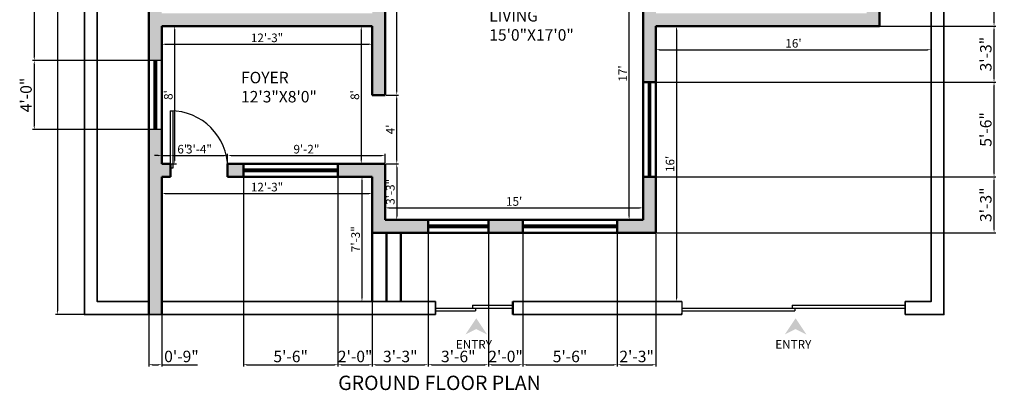
# Model space of a CAD drawing. Units: inches. Extents: x 2442 to 3851, y 589 to 2836.
# Tile 13 of 22: x 2448 to 3136, y 2138 to 2397. Entities that reach past the tile are written whole.
import ezdxf

# ---------------------------------------------------------------- set-up
doc = ezdxf.new("R2010")
doc.units = ezdxf.units.IN
for name, color, linetype, lineweight in [('A-ANNO-DIMS', 2, 'Continuous', 18), ('A-ANNO-SYMB', 1, 'Continuous', 18), ('A-ANNO-TEXT', 7, 'Continuous', 18), ('A-AREA-IDEN', 7, 'Continuous', 18), ('A-DOOR', 4, 'Continuous', 25), ('A-GLAZ', 1, 'Continuous', 25), ('A-WALL', 7, 'Continuous', 50), ('A-WALL-PATT', 8, 'Continuous', 13), ('C-PROP', 7, 'Continuous', 35)]:
    doc.layers.add(name, color=color, linetype=linetype, lineweight=lineweight)
doc.styles.get("Standard").update_dxf_attribs({"font": 'arial.ttf'})
doc.dimstyles.new('ISO-25', dxfattribs={"dimtxt": 8, "dimasz": 2.5, "dimexe": 1.25, "dimexo": 0.625, "dimtad": 1, "dimlunit": 3, "dimtxsty": 'Standard', "dimcen": 2.5, "dimadec": 0, "dimazin": 0, "dimtfac": 1, "dimtmove": 0, "dimatfit": 3, "dimfxl": 1, "dimarcsym": 0})

# ---------------------------------------------------------------- blocks, each defined once
blk = doc.blocks.new('*U22')
for p, q in [((0, 0), (0, -6)), ((40, 0), (40, -6))]:
    blk.add_line(p, q)
blk.add_lwpolyline([(0, 0), (0, 40), (1.75, 40), (1.75, 0)], close=True)
blk.add_arc((0, 0), 40, 0, 90)
blk = doc.blocks.new('*D36')
at = {"layer": 'A-ANNO-DIMS', "color": 0, "lineweight": -2, "transparency": 16777216}
for p, q in [((2492.97, 2791.21), (2473.47, 2791.21)), ((2474.72, 2788.71), (2474.72, 2193.71)), ((2492.97, 2191.21), (2473.47, 2191.21))]:
    blk.add_line(p, q, dxfattribs=at)
at = {"layer": 'A-ANNO-DIMS', "color": 0, "transparency": 16777216}
for points in [[(2474.3, 2788.71), (2475.14, 2788.71), (2474.72, 2791.21)], [(2474.3, 2193.71), (2475.14, 2193.71), (2474.72, 2191.21)]]:
    blk.add_solid(points, dxfattribs=at)
at = {"layer": 'Defpoints', "color": 0, "transparency": 16777216}
for p in [(2493.6, 2791.21), (2474.72, 2191.21), (2493.6, 2191.21)]:
    blk.add_point(p, dxfattribs=at)
at = {"layer": 'A-ANNO-DIMS', "color": 0, "transparency": 16777216, "insert": (2470.01, 2491.21), "char_height": 8, "attachment_point": 5, "rotation": 90}
blk.add_mtext("50'", dxfattribs=at)
blk = doc.blocks.new('*D54')
at = {"layer": 'A-ANNO-DIMS', "color": 0, "lineweight": -2, "transparency": 16777216}
for p, q in [((2703.6, 2257.83), (2703.6, 2266.79)), ((2706.1, 2265.54), (2881.1, 2265.54)), ((2883.6, 2257.83), (2883.6, 2266.79))]:
    blk.add_line(p, q, dxfattribs=at)
at = {"layer": 'A-ANNO-DIMS', "color": 0, "transparency": 16777216}
for points in [[(2706.1, 2265.96), (2706.1, 2265.13), (2703.6, 2265.54)], [(2881.1, 2265.96), (2881.1, 2265.13), (2883.6, 2265.54)]]:
    blk.add_solid(points, dxfattribs=at)
at = {"layer": 'Defpoints', "color": 0, "transparency": 16777216}
for p in [(2883.6, 2265.54), (2703.6, 2257.21), (2883.6, 2257.21)]:
    blk.add_point(p, dxfattribs=at)
at = {"layer": 'A-ANNO-DIMS', "color": 0, "transparency": 16777216, "insert": (2793.6, 2269.23), "char_height": 6, "attachment_point": 5}
blk.add_mtext("15'", dxfattribs=at)
blk = doc.blocks.new('*D55')
at = {"layer": 'A-ANNO-DIMS', "color": 0, "lineweight": -2, "transparency": 16777216}
for p, q in [((2882.97, 2461.21), (2872.6, 2461.21)), ((2873.85, 2259.71), (2873.85, 2458.71)), ((2882.97, 2257.21), (2872.6, 2257.21))]:
    blk.add_line(p, q, dxfattribs=at)
at = {"layer": 'A-ANNO-DIMS', "color": 0, "transparency": 16777216}
for points in [[(2873.44, 2458.71), (2874.27, 2458.71), (2873.85, 2461.21)], [(2873.44, 2259.71), (2874.27, 2259.71), (2873.85, 2257.21)]]:
    blk.add_solid(points, dxfattribs=at)
at = {"layer": 'Defpoints', "color": 0, "transparency": 16777216}
for p in [(2873.85, 2461.21), (2883.6, 2461.21), (2883.6, 2257.21)]:
    blk.add_point(p, dxfattribs=at)
at = {"layer": 'A-ANNO-DIMS', "color": 0, "transparency": 16777216, "insert": (2870.22, 2359.21), "char_height": 6, "attachment_point": 5, "rotation": 90}
blk.add_mtext("17'", dxfattribs=at)
blk = doc.blocks.new('*D58')
at = {"layer": 'A-ANNO-DIMS', "color": 0, "lineweight": -2, "transparency": 16777216}
for p, q in [((2547.6, 2391.58), (2547.6, 2378.36)), ((2694.6, 2391.58), (2694.6, 2378.36)), ((2550.1, 2379.61), (2692.1, 2379.61))]:
    blk.add_line(p, q, dxfattribs=at)
at = {"layer": 'A-ANNO-DIMS', "color": 0, "transparency": 16777216}
for points in [[(2550.1, 2380.03), (2550.1, 2379.19), (2547.6, 2379.61)], [(2692.1, 2380.03), (2692.1, 2379.19), (2694.6, 2379.61)]]:
    blk.add_solid(points, dxfattribs=at)
at = {"layer": 'Defpoints', "color": 0, "transparency": 16777216}
for p in [(2547.6, 2392.21), (2694.6, 2392.21), (2694.6, 2379.61)]:
    blk.add_point(p, dxfattribs=at)
at = {"layer": 'A-ANNO-DIMS', "color": 0, "transparency": 16777216, "insert": (2621.1, 2383.3), "char_height": 6, "attachment_point": 5}
blk.add_mtext('12\'-3"', dxfattribs=at)
blk = doc.blocks.new('*D59')
at = {"layer": 'A-ANNO-DIMS', "color": 0, "lineweight": -2, "transparency": 16777216}
for p, q in [((2693.97, 2392.21), (2685.61, 2392.21)), ((2686.86, 2389.71), (2686.86, 2298.71)), ((2693.97, 2296.21), (2685.61, 2296.21))]:
    blk.add_line(p, q, dxfattribs=at)
at = {"layer": 'A-ANNO-DIMS', "color": 0, "transparency": 16777216}
for points in [[(2686.44, 2389.71), (2687.27, 2389.71), (2686.86, 2392.21)], [(2686.44, 2298.71), (2687.27, 2298.71), (2686.86, 2296.21)]]:
    blk.add_solid(points, dxfattribs=at)
at = {"layer": 'Defpoints', "color": 0, "transparency": 16777216}
for p in [(2694.6, 2392.21), (2686.86, 2296.21), (2694.6, 2296.21)]:
    blk.add_point(p, dxfattribs=at)
at = {"layer": 'A-ANNO-DIMS', "color": 0, "transparency": 16777216, "insert": (2683.17, 2344.21), "char_height": 6, "attachment_point": 5, "rotation": 90}
blk.add_mtext("8'", dxfattribs=at)
blk = doc.blocks.new('*D77')
at = {"layer": 'A-ANNO-DIMS', "color": 0, "lineweight": -2, "transparency": 16777216}
for p, q in [((2548.22, 2392.21), (2557.88, 2392.21)), ((2556.63, 2298.71), (2556.63, 2389.71)), ((2548.22, 2296.21), (2557.88, 2296.21))]:
    blk.add_line(p, q, dxfattribs=at)
at = {"layer": 'A-ANNO-DIMS', "color": 0, "transparency": 16777216}
for points in [[(2556.21, 2389.71), (2557.05, 2389.71), (2556.63, 2392.21)], [(2556.21, 2298.71), (2557.05, 2298.71), (2556.63, 2296.21)]]:
    blk.add_solid(points, dxfattribs=at)
at = {"layer": 'Defpoints', "color": 0, "transparency": 16777216}
for p in [(2547.6, 2392.21), (2556.63, 2392.21), (2547.6, 2296.21)]:
    blk.add_point(p, dxfattribs=at)
at = {"layer": 'A-ANNO-DIMS', "color": 0, "transparency": 16777216, "insert": (2552.94, 2344.21), "char_height": 6, "attachment_point": 5, "rotation": 90}
blk.add_mtext("8'", dxfattribs=at)
blk = doc.blocks.new('*D78')
at = {"layer": 'A-ANNO-DIMS', "color": 0, "lineweight": -2, "transparency": 16777216}
for p, q in [((2547.6, 2296.83), (2547.6, 2303.24)), ((2553.6, 2296.83), (2553.6, 2303.24)), ((2545.1, 2301.99), (2542.6, 2301.99)), ((2547.6, 2301.99), (2553.6, 2301.99)), ((2556.1, 2301.99), (2566.78, 2301.99))]:
    blk.add_line(p, q, dxfattribs=at)
at = {"layer": 'A-ANNO-DIMS', "color": 0, "transparency": 16777216}
for points in [[(2545.1, 2302.41), (2545.1, 2301.58), (2547.6, 2301.99)], [(2556.1, 2302.41), (2556.1, 2301.58), (2553.6, 2301.99)]]:
    blk.add_solid(points, dxfattribs=at)
at = {"layer": 'Defpoints', "color": 0, "transparency": 16777216}
for p in [(2547.6, 2296.21), (2553.6, 2301.99), (2553.6, 2296.21)]:
    blk.add_point(p, dxfattribs=at)
at = {"layer": 'A-ANNO-DIMS', "color": 0, "transparency": 16777216, "insert": (2562.69, 2305.68), "char_height": 6, "attachment_point": 5}
blk.add_mtext('6"', dxfattribs=at)
blk = doc.blocks.new('*D79')
at = {"layer": 'A-ANNO-DIMS', "color": 0, "lineweight": -2, "transparency": 16777216}
for p, q in [((2553.6, 2296.83), (2553.6, 2303.24)), ((2593.6, 2296.83), (2593.6, 2303.24)), ((2556.1, 2301.99), (2591.1, 2301.99))]:
    blk.add_line(p, q, dxfattribs=at)
at = {"layer": 'A-ANNO-DIMS', "color": 0, "transparency": 16777216}
for points in [[(2556.1, 2302.41), (2556.1, 2301.58), (2553.6, 2301.99)], [(2591.1, 2302.41), (2591.1, 2301.58), (2593.6, 2301.99)]]:
    blk.add_solid(points, dxfattribs=at)
at = {"layer": 'Defpoints', "color": 0, "transparency": 16777216}
for p in [(2553.6, 2296.21), (2593.6, 2301.99), (2593.6, 2296.21)]:
    blk.add_point(p, dxfattribs=at)
at = {"layer": 'A-ANNO-DIMS', "color": 0, "transparency": 16777216, "insert": (2573.6, 2305.68), "char_height": 6, "attachment_point": 5}
blk.add_mtext('3\'-4"', dxfattribs=at)
blk = doc.blocks.new('*D80')
at = {"layer": 'A-ANNO-DIMS', "color": 0, "lineweight": -2, "transparency": 16777216}
for p, q in [((2593.6, 2296.83), (2593.6, 2303.24)), ((2703.6, 2296.83), (2703.6, 2303.24)), ((2596.1, 2301.99), (2701.1, 2301.99))]:
    blk.add_line(p, q, dxfattribs=at)
at = {"layer": 'A-ANNO-DIMS', "color": 0, "transparency": 16777216}
for points in [[(2596.1, 2302.41), (2596.1, 2301.58), (2593.6, 2301.99)], [(2701.1, 2302.41), (2701.1, 2301.58), (2703.6, 2301.99)]]:
    blk.add_solid(points, dxfattribs=at)
at = {"layer": 'Defpoints', "color": 0, "transparency": 16777216}
for p in [(2593.6, 2296.21), (2703.6, 2301.99), (2703.6, 2296.21)]:
    blk.add_point(p, dxfattribs=at)
at = {"layer": 'A-ANNO-DIMS', "color": 0, "transparency": 16777216, "insert": (2648.6, 2305.68), "char_height": 6, "attachment_point": 5}
blk.add_mtext('9\'-2"', dxfattribs=at)
blk = doc.blocks.new('*D81')
at = {"layer": 'A-ANNO-DIMS', "color": 0, "lineweight": -2, "transparency": 16777216}
for p, q in [((2704.22, 2296.21), (2712.89, 2296.21)), ((2711.64, 2293.71), (2711.64, 2259.71)), ((2704.22, 2257.21), (2712.89, 2257.21))]:
    blk.add_line(p, q, dxfattribs=at)
at = {"layer": 'A-ANNO-DIMS', "color": 0, "transparency": 16777216}
for points in [[(2711.22, 2293.71), (2712.05, 2293.71), (2711.64, 2296.21)], [(2711.22, 2259.71), (2712.05, 2259.71), (2711.64, 2257.21)]]:
    blk.add_solid(points, dxfattribs=at)
at = {"layer": 'Defpoints', "color": 0, "transparency": 16777216}
for p in [(2703.6, 2296.21), (2703.6, 2257.21), (2711.64, 2257.21)]:
    blk.add_point(p, dxfattribs=at)
at = {"layer": 'A-ANNO-DIMS', "color": 0, "transparency": 16777216, "insert": (2707.95, 2276.71), "char_height": 6, "attachment_point": 5, "rotation": 90}
blk.add_mtext('3\'-3"', dxfattribs=at)
blk = doc.blocks.new('*D82')
at = {"layer": 'A-ANNO-DIMS', "color": 0, "lineweight": -2, "transparency": 16777216}
for p, q in [((2704.22, 2344.21), (2712.89, 2344.21)), ((2711.64, 2298.71), (2711.64, 2341.71)), ((2704.22, 2296.21), (2712.89, 2296.21))]:
    blk.add_line(p, q, dxfattribs=at)
at = {"layer": 'A-ANNO-DIMS', "color": 0, "transparency": 16777216}
for points in [[(2711.22, 2341.71), (2712.05, 2341.71), (2711.64, 2344.21)], [(2711.22, 2298.71), (2712.05, 2298.71), (2711.64, 2296.21)]]:
    blk.add_solid(points, dxfattribs=at)
at = {"layer": 'Defpoints', "color": 0, "transparency": 16777216}
for p in [(2703.6, 2344.21), (2711.64, 2344.21), (2703.6, 2296.21)]:
    blk.add_point(p, dxfattribs=at)
at = {"layer": 'A-ANNO-DIMS', "color": 0, "transparency": 16777216, "insert": (2708.01, 2320.21), "char_height": 6, "attachment_point": 5, "rotation": 90}
blk.add_mtext("4'", dxfattribs=at)
blk = doc.blocks.new('*D83')
at = {"layer": 'A-ANNO-DIMS', "color": 0, "lineweight": -2, "transparency": 16777216}
for p, q in [((2704.22, 2506.21), (2712.89, 2506.21)), ((2711.64, 2346.71), (2711.64, 2503.71)), ((2704.22, 2344.21), (2712.89, 2344.21))]:
    blk.add_line(p, q, dxfattribs=at)
at = {"layer": 'A-ANNO-DIMS', "color": 0, "transparency": 16777216}
for points in [[(2711.22, 2503.71), (2712.05, 2503.71), (2711.64, 2506.21)], [(2711.22, 2346.71), (2712.05, 2346.71), (2711.64, 2344.21)]]:
    blk.add_solid(points, dxfattribs=at)
at = {"layer": 'Defpoints', "color": 0, "transparency": 16777216}
for p in [(2703.6, 2506.21), (2711.64, 2506.21), (2703.6, 2344.21)]:
    blk.add_point(p, dxfattribs=at)
at = {"layer": 'A-ANNO-DIMS', "color": 0, "transparency": 16777216, "insert": (2707.95, 2425.21), "char_height": 6, "attachment_point": 5, "rotation": 90}
blk.add_mtext('13\'-6"', dxfattribs=at)
blk = doc.blocks.new('*D89')
at = {"layer": 'A-ANNO-DIMS', "color": 0, "lineweight": -2, "transparency": 16777216}
for p, q in [((2892.6, 2391.58), (2892.6, 2374.53)), ((3084.6, 2391.58), (3084.6, 2374.53)), ((2895.1, 2375.78), (3082.1, 2375.78))]:
    blk.add_line(p, q, dxfattribs=at)
at = {"layer": 'A-ANNO-DIMS', "color": 0, "transparency": 16777216}
for points in [[(2895.1, 2376.2), (2895.1, 2375.37), (2892.6, 2375.78)], [(3082.1, 2376.2), (3082.1, 2375.37), (3084.6, 2375.78)]]:
    blk.add_solid(points, dxfattribs=at)
at = {"layer": 'Defpoints', "color": 0, "transparency": 16777216}
for p in [(2892.6, 2392.21), (3084.6, 2392.21), (3084.6, 2375.78)]:
    blk.add_point(p, dxfattribs=at)
at = {"layer": 'A-ANNO-DIMS', "color": 0, "transparency": 16777216, "insert": (2988.6, 2379.47), "char_height": 6, "attachment_point": 5}
blk.add_mtext("16'", dxfattribs=at)
blk = doc.blocks.new('*D90')
at = {"layer": 'A-ANNO-DIMS', "color": 0, "lineweight": -2, "transparency": 16777216}
for p, q in [((2893.22, 2392.21), (2908.16, 2392.21)), ((2906.91, 2389.71), (2906.91, 2202.71)), ((2893.22, 2200.21), (2908.16, 2200.21))]:
    blk.add_line(p, q, dxfattribs=at)
at = {"layer": 'A-ANNO-DIMS', "color": 0, "transparency": 16777216}
for points in [[(2906.5, 2389.71), (2907.33, 2389.71), (2906.91, 2392.21)], [(2906.5, 2202.71), (2907.33, 2202.71), (2906.91, 2200.21)]]:
    blk.add_solid(points, dxfattribs=at)
at = {"layer": 'Defpoints', "color": 0, "transparency": 16777216}
for p in [(2892.6, 2392.21), (2892.6, 2200.21), (2906.91, 2200.21)]:
    blk.add_point(p, dxfattribs=at)
at = {"layer": 'A-ANNO-DIMS', "color": 0, "transparency": 16777216, "insert": (2903.22, 2296.21), "char_height": 6, "attachment_point": 5, "rotation": 90}
blk.add_mtext("16'", dxfattribs=at)
blk = doc.blocks.new('*D91')
at = {"layer": 'A-ANNO-DIMS', "color": 0, "lineweight": -2, "transparency": 16777216}
for p, q in [((2694.6, 2286.58), (2694.6, 2274.29)), ((2547.6, 2277.87), (2547.6, 2274.29)), ((2550.1, 2275.54), (2692.1, 2275.54))]:
    blk.add_line(p, q, dxfattribs=at)
at = {"layer": 'A-ANNO-DIMS', "color": 0, "transparency": 16777216}
for points in [[(2550.1, 2275.95), (2550.1, 2275.12), (2547.6, 2275.54)], [(2692.1, 2275.95), (2692.1, 2275.12), (2694.6, 2275.54)]]:
    blk.add_solid(points, dxfattribs=at)
at = {"layer": 'Defpoints', "color": 0, "transparency": 16777216}
for p in [(2694.6, 2287.21), (2547.6, 2278.49), (2694.6, 2275.54)]:
    blk.add_point(p, dxfattribs=at)
at = {"layer": 'A-ANNO-DIMS', "color": 0, "transparency": 16777216, "insert": (2621.1, 2279.23), "char_height": 6, "attachment_point": 5}
blk.add_mtext('12\'-3"', dxfattribs=at)
blk = doc.blocks.new('*D92')
at = {"layer": 'A-ANNO-DIMS', "color": 0, "lineweight": -2, "transparency": 16777216}
for p, q in [((2693.97, 2287.21), (2686.12, 2287.21)), ((2687.37, 2284.71), (2687.37, 2202.71)), ((2693.97, 2200.21), (2686.12, 2200.21))]:
    blk.add_line(p, q, dxfattribs=at)
at = {"layer": 'A-ANNO-DIMS', "color": 0, "transparency": 16777216}
for points in [[(2686.95, 2284.71), (2687.78, 2284.71), (2687.37, 2287.21)], [(2686.95, 2202.71), (2687.78, 2202.71), (2687.37, 2200.21)]]:
    blk.add_solid(points, dxfattribs=at)
at = {"layer": 'Defpoints', "color": 0, "transparency": 16777216}
for p in [(2694.6, 2287.21), (2687.37, 2200.21), (2694.6, 2200.21)]:
    blk.add_point(p, dxfattribs=at)
at = {"layer": 'A-ANNO-DIMS', "color": 0, "transparency": 16777216, "insert": (2683.68, 2243.71), "char_height": 6, "attachment_point": 5, "rotation": 90}
blk.add_mtext('7\'-3"', dxfattribs=at)
blk = doc.blocks.new('*D191')
at = {"layer": 'A-ANNO-DIMS', "color": 0, "lineweight": -2, "transparency": 16777216}
for p, q in [((3128.6, 2426.71), (3128.6, 2476.72)), ((3049.22, 2426.71), (3129.85, 2426.71)), ((3128.6, 2394.71), (3128.6, 2424.21)), ((3049.22, 2392.21), (3129.85, 2392.21))]:
    blk.add_line(p, q, dxfattribs=at)
at = {"layer": 'A-ANNO-DIMS', "color": 0, "transparency": 16777216}
for points in [[(3128.18, 2424.21), (3129.02, 2424.21), (3128.6, 2426.71)], [(3128.18, 2394.71), (3129.02, 2394.71), (3128.6, 2392.21)]]:
    blk.add_solid(points, dxfattribs=at)
at = {"layer": 'Defpoints', "color": 0, "transparency": 16777216}
for p in [(3048.6, 2426.71), (3128.6, 2426.71), (3048.6, 2392.21)]:
    blk.add_point(p, dxfattribs=at)
at = {"layer": 'A-ANNO-DIMS', "color": 0, "transparency": 16777216, "insert": (3123.84, 2452.96), "char_height": 8, "attachment_point": 5, "rotation": 90}
blk.add_mtext('2\'-10 1/2"', dxfattribs=at)
blk = doc.blocks.new('*D202')
at = {"layer": 'A-ANNO-DIMS', "color": 0, "lineweight": -2, "transparency": 16777216}
for p, q in [((2537.97, 2473.21), (2457.35, 2473.21)), ((2458.6, 2470.71), (2458.6, 2370.71)), ((2537.97, 2368.21), (2457.35, 2368.21))]:
    blk.add_line(p, q, dxfattribs=at)
at = {"layer": 'A-ANNO-DIMS', "color": 0, "transparency": 16777216}
for points in [[(2458.18, 2470.71), (2459.02, 2470.71), (2458.6, 2473.21)], [(2458.18, 2370.71), (2459.02, 2370.71), (2458.6, 2368.21)]]:
    blk.add_solid(points, dxfattribs=at)
at = {"layer": 'Defpoints', "color": 0, "transparency": 16777216}
for p in [(2538.6, 2473.21), (2458.6, 2368.21), (2538.6, 2368.21)]:
    blk.add_point(p, dxfattribs=at)
at = {"layer": 'A-ANNO-DIMS', "color": 0, "transparency": 16777216, "insert": (2453.89, 2420.71), "char_height": 8, "attachment_point": 5, "rotation": 90}
blk.add_mtext('8\'-9"', dxfattribs=at)
blk = doc.blocks.new('*D203')
at = {"layer": 'A-ANNO-DIMS', "color": 0, "lineweight": -2, "transparency": 16777216}
for p, q in [((2537.97, 2368.21), (2457.35, 2368.21)), ((2458.6, 2365.71), (2458.6, 2322.71)), ((2537.97, 2320.21), (2457.35, 2320.21))]:
    blk.add_line(p, q, dxfattribs=at)
at = {"layer": 'A-ANNO-DIMS', "color": 0, "transparency": 16777216}
for points in [[(2458.18, 2365.71), (2459.02, 2365.71), (2458.6, 2368.21)], [(2458.18, 2322.71), (2459.02, 2322.71), (2458.6, 2320.21)]]:
    blk.add_solid(points, dxfattribs=at)
at = {"layer": 'Defpoints', "color": 0, "transparency": 16777216}
for p in [(2538.6, 2368.21), (2458.6, 2320.21), (2538.6, 2320.21)]:
    blk.add_point(p, dxfattribs=at)
at = {"layer": 'A-ANNO-DIMS', "color": 0, "transparency": 16777216, "insert": (2453.89, 2344.21), "char_height": 8, "attachment_point": 5, "rotation": 90}
blk.add_mtext('4\'-0"', dxfattribs=at)
blk = doc.blocks.new('*D204')
at = {"layer": 'A-ANNO-DIMS', "color": 0, "lineweight": -2, "transparency": 16777216}
for p, q in [((2604.6, 2286.58), (2604.6, 2154.96)), ((2670.6, 2286.58), (2670.6, 2154.96)), ((2607.1, 2156.21), (2668.1, 2156.21))]:
    blk.add_line(p, q, dxfattribs=at)
at = {"layer": 'A-ANNO-DIMS', "color": 0, "transparency": 16777216}
for points in [[(2607.1, 2156.62), (2607.1, 2155.79), (2604.6, 2156.21)], [(2668.1, 2156.62), (2668.1, 2155.79), (2670.6, 2156.21)]]:
    blk.add_solid(points, dxfattribs=at)
at = {"layer": 'Defpoints', "color": 0, "transparency": 16777216}
for p in [(2604.6, 2287.21), (2670.6, 2287.21), (2670.6, 2156.21)]:
    blk.add_point(p, dxfattribs=at)
at = {"layer": 'A-ANNO-DIMS', "color": 0, "transparency": 16777216, "insert": (2637.6, 2160.92), "char_height": 8, "attachment_point": 5}
blk.add_mtext('5\'-6"', dxfattribs=at)
blk = doc.blocks.new('*D205')
at = {"layer": 'A-ANNO-DIMS', "color": 0, "lineweight": -2, "transparency": 16777216}
for p, q in [((2670.6, 2286.58), (2670.6, 2154.96)), ((2694.6, 2286.58), (2694.6, 2154.96)), ((2673.1, 2156.21), (2692.1, 2156.21))]:
    blk.add_line(p, q, dxfattribs=at)
at = {"layer": 'A-ANNO-DIMS', "color": 0, "transparency": 16777216}
for points in [[(2673.1, 2156.62), (2673.1, 2155.79), (2670.6, 2156.21)], [(2692.1, 2156.62), (2692.1, 2155.79), (2694.6, 2156.21)]]:
    blk.add_solid(points, dxfattribs=at)
at = {"layer": 'Defpoints', "color": 0, "transparency": 16777216}
for p in [(2670.6, 2287.21), (2694.6, 2287.21), (2694.6, 2156.21)]:
    blk.add_point(p, dxfattribs=at)
at = {"layer": 'A-ANNO-DIMS', "color": 0, "transparency": 16777216, "insert": (2682.6, 2160.92), "char_height": 8, "attachment_point": 5}
blk.add_mtext('2\'-0"', dxfattribs=at)
blk = doc.blocks.new('*D206')
at = {"layer": 'A-ANNO-DIMS', "color": 0, "lineweight": -2, "transparency": 16777216}
for p, q in [((2694.6, 2247.58), (2694.6, 2154.96)), ((2733.6, 2247.58), (2733.6, 2154.96)), ((2697.1, 2156.21), (2731.1, 2156.21))]:
    blk.add_line(p, q, dxfattribs=at)
at = {"layer": 'A-ANNO-DIMS', "color": 0, "transparency": 16777216}
for points in [[(2697.1, 2156.62), (2697.1, 2155.79), (2694.6, 2156.21)], [(2731.1, 2156.62), (2731.1, 2155.79), (2733.6, 2156.21)]]:
    blk.add_solid(points, dxfattribs=at)
at = {"layer": 'Defpoints', "color": 0, "transparency": 16777216}
for p in [(2694.6, 2248.21), (2733.6, 2248.21), (2733.6, 2156.21)]:
    blk.add_point(p, dxfattribs=at)
at = {"layer": 'A-ANNO-DIMS', "color": 0, "transparency": 16777216, "insert": (2714.1, 2160.92), "char_height": 8, "attachment_point": 5}
blk.add_mtext('3\'-3"', dxfattribs=at)
blk = doc.blocks.new('*D207')
at = {"layer": 'A-ANNO-DIMS', "color": 0, "lineweight": -2, "transparency": 16777216}
for p, q in [((2733.6, 2247.58), (2733.6, 2154.96)), ((2775.6, 2247.58), (2775.6, 2154.96)), ((2736.1, 2156.21), (2773.1, 2156.21))]:
    blk.add_line(p, q, dxfattribs=at)
at = {"layer": 'A-ANNO-DIMS', "color": 0, "transparency": 16777216}
for points in [[(2736.1, 2156.62), (2736.1, 2155.79), (2733.6, 2156.21)], [(2773.1, 2156.62), (2773.1, 2155.79), (2775.6, 2156.21)]]:
    blk.add_solid(points, dxfattribs=at)
at = {"layer": 'Defpoints', "color": 0, "transparency": 16777216}
for p in [(2733.6, 2248.21), (2775.6, 2248.21), (2775.6, 2156.21)]:
    blk.add_point(p, dxfattribs=at)
at = {"layer": 'A-ANNO-DIMS', "color": 0, "transparency": 16777216, "insert": (2754.6, 2160.92), "char_height": 8, "attachment_point": 5}
blk.add_mtext('3\'-6"', dxfattribs=at)
blk = doc.blocks.new('*D208')
at = {"layer": 'A-ANNO-DIMS', "color": 0, "lineweight": -2, "transparency": 16777216}
for p, q in [((2775.6, 2247.58), (2775.6, 2154.96)), ((2799.6, 2247.58), (2799.6, 2154.96)), ((2778.1, 2156.21), (2797.1, 2156.21))]:
    blk.add_line(p, q, dxfattribs=at)
at = {"layer": 'A-ANNO-DIMS', "color": 0, "transparency": 16777216}
for points in [[(2778.1, 2156.62), (2778.1, 2155.79), (2775.6, 2156.21)], [(2797.1, 2156.62), (2797.1, 2155.79), (2799.6, 2156.21)]]:
    blk.add_solid(points, dxfattribs=at)
at = {"layer": 'Defpoints', "color": 0, "transparency": 16777216}
for p in [(2775.6, 2248.21), (2799.6, 2248.21), (2799.6, 2156.21)]:
    blk.add_point(p, dxfattribs=at)
at = {"layer": 'A-ANNO-DIMS', "color": 0, "transparency": 16777216, "insert": (2787.6, 2160.92), "char_height": 8, "attachment_point": 5}
blk.add_mtext('2\'-0"', dxfattribs=at)
blk = doc.blocks.new('*D209')
at = {"layer": 'A-ANNO-DIMS', "color": 0, "lineweight": -2, "transparency": 16777216}
for p, q in [((2799.6, 2247.58), (2799.6, 2154.96)), ((2865.6, 2247.58), (2865.6, 2154.96)), ((2802.1, 2156.21), (2863.1, 2156.21))]:
    blk.add_line(p, q, dxfattribs=at)
at = {"layer": 'A-ANNO-DIMS', "color": 0, "transparency": 16777216}
for points in [[(2802.1, 2156.62), (2802.1, 2155.79), (2799.6, 2156.21)], [(2863.1, 2156.62), (2863.1, 2155.79), (2865.6, 2156.21)]]:
    blk.add_solid(points, dxfattribs=at)
at = {"layer": 'Defpoints', "color": 0, "transparency": 16777216}
for p in [(2799.6, 2248.21), (2865.6, 2248.21), (2865.6, 2156.21)]:
    blk.add_point(p, dxfattribs=at)
at = {"layer": 'A-ANNO-DIMS', "color": 0, "transparency": 16777216, "insert": (2832.6, 2160.92), "char_height": 8, "attachment_point": 5}
blk.add_mtext('5\'-6"', dxfattribs=at)
blk = doc.blocks.new('*D210')
at = {"layer": 'A-ANNO-DIMS', "color": 0, "lineweight": -2, "transparency": 16777216}
for p, q in [((2865.6, 2247.58), (2865.6, 2154.96)), ((2892.6, 2247.58), (2892.6, 2154.96)), ((2868.1, 2156.21), (2890.1, 2156.21))]:
    blk.add_line(p, q, dxfattribs=at)
at = {"layer": 'A-ANNO-DIMS', "color": 0, "transparency": 16777216}
for points in [[(2868.1, 2156.62), (2868.1, 2155.79), (2865.6, 2156.21)], [(2890.1, 2156.62), (2890.1, 2155.79), (2892.6, 2156.21)]]:
    blk.add_solid(points, dxfattribs=at)
at = {"layer": 'Defpoints', "color": 0, "transparency": 16777216}
for p in [(2865.6, 2248.21), (2892.6, 2248.21), (2892.6, 2156.21)]:
    blk.add_point(p, dxfattribs=at)
at = {"layer": 'A-ANNO-DIMS', "color": 0, "transparency": 16777216, "insert": (2879.1, 2160.92), "char_height": 8, "attachment_point": 5}
blk.add_mtext('2\'-3"', dxfattribs=at)
blk = doc.blocks.new('*D211')
at = {"layer": 'A-ANNO-DIMS', "color": 0, "lineweight": -2, "transparency": 16777216}
for p, q in [((2893.22, 2287.21), (3129.85, 2287.21)), ((3128.6, 2250.71), (3128.6, 2284.71)), ((2893.22, 2248.21), (3129.85, 2248.21))]:
    blk.add_line(p, q, dxfattribs=at)
at = {"layer": 'A-ANNO-DIMS', "color": 0, "transparency": 16777216}
for points in [[(3128.18, 2284.71), (3129.02, 2284.71), (3128.6, 2287.21)], [(3128.18, 2250.71), (3129.02, 2250.71), (3128.6, 2248.21)]]:
    blk.add_solid(points, dxfattribs=at)
at = {"layer": 'Defpoints', "color": 0, "transparency": 16777216}
for p in [(2892.6, 2287.21), (3128.6, 2287.21), (2892.6, 2248.21)]:
    blk.add_point(p, dxfattribs=at)
at = {"layer": 'A-ANNO-DIMS', "color": 0, "transparency": 16777216, "insert": (3123.89, 2267.71), "char_height": 8, "attachment_point": 5, "rotation": 90}
blk.add_mtext('3\'-3"', dxfattribs=at)
blk = doc.blocks.new('*D212')
at = {"layer": 'A-ANNO-DIMS', "color": 0, "lineweight": -2, "transparency": 16777216}
for p, q in [((2893.22, 2353.21), (3129.85, 2353.21)), ((3128.6, 2289.71), (3128.6, 2350.71)), ((2893.22, 2287.21), (3129.85, 2287.21))]:
    blk.add_line(p, q, dxfattribs=at)
at = {"layer": 'A-ANNO-DIMS', "color": 0, "transparency": 16777216}
for points in [[(3128.18, 2350.71), (3129.02, 2350.71), (3128.6, 2353.21)], [(3128.18, 2289.71), (3129.02, 2289.71), (3128.6, 2287.21)]]:
    blk.add_solid(points, dxfattribs=at)
at = {"layer": 'Defpoints', "color": 0, "transparency": 16777216}
for p in [(2892.6, 2353.21), (3128.6, 2353.21), (2892.6, 2287.21)]:
    blk.add_point(p, dxfattribs=at)
at = {"layer": 'A-ANNO-DIMS', "color": 0, "transparency": 16777216, "insert": (3123.89, 2320.21), "char_height": 8, "attachment_point": 5, "rotation": 90}
blk.add_mtext('5\'-6"', dxfattribs=at)
blk = doc.blocks.new('*D213')
at = {"layer": 'A-ANNO-DIMS', "color": 0, "lineweight": -2, "transparency": 16777216}
for p, q in [((2893.22, 2392.21), (3129.85, 2392.21)), ((3128.6, 2355.71), (3128.6, 2389.71)), ((2893.22, 2353.21), (3129.85, 2353.21))]:
    blk.add_line(p, q, dxfattribs=at)
at = {"layer": 'A-ANNO-DIMS', "color": 0, "transparency": 16777216}
for points in [[(3128.18, 2389.71), (3129.02, 2389.71), (3128.6, 2392.21)], [(3128.18, 2355.71), (3129.02, 2355.71), (3128.6, 2353.21)]]:
    blk.add_solid(points, dxfattribs=at)
at = {"layer": 'Defpoints', "color": 0, "transparency": 16777216}
for p in [(2892.6, 2392.21), (3128.6, 2392.21), (2892.6, 2353.21)]:
    blk.add_point(p, dxfattribs=at)
at = {"layer": 'A-ANNO-DIMS', "color": 0, "transparency": 16777216, "insert": (3123.89, 2372.71), "char_height": 8, "attachment_point": 5, "rotation": 90}
blk.add_mtext('3\'-3"', dxfattribs=at)
blk = doc.blocks.new('*D214')
at = {"layer": 'A-ANNO-DIMS', "color": 0, "lineweight": -2, "transparency": 16777216}
for p, q in [((2538.6, 2190.58), (2538.6, 2154.96)), ((2547.6, 2190.58), (2547.6, 2154.96)), ((2541.1, 2156.21), (2545.1, 2156.21)), ((2547.6, 2156.21), (2572.61, 2156.21))]:
    blk.add_line(p, q, dxfattribs=at)
at = {"layer": 'A-ANNO-DIMS', "color": 0, "transparency": 16777216}
for points in [[(2541.1, 2156.62), (2541.1, 2155.79), (2538.6, 2156.21)], [(2545.1, 2156.62), (2545.1, 2155.79), (2547.6, 2156.21)]]:
    blk.add_solid(points, dxfattribs=at)
at = {"layer": 'Defpoints', "color": 0, "transparency": 16777216}
for p in [(2538.6, 2191.21), (2547.6, 2191.21), (2547.6, 2156.21)]:
    blk.add_point(p, dxfattribs=at)
at = {"layer": 'A-ANNO-DIMS', "color": 0, "transparency": 16777216, "insert": (2561.36, 2160.92), "char_height": 8, "attachment_point": 5}
blk.add_mtext('0\'-9"', dxfattribs=at)

msp = doc.modelspace()

# ---------------------------------------------------------------- hatches: boundary and pattern name
at = {"layer": 'A-ANNO-SYMB'}
h = msp.add_hatch(color=256, dxfattribs=at)
h.dxf.hatch_style = 1
h.paths.add_polyline_path([(2767.136, 2188.599), (2759.585, 2177.274), (2767.136, 2181.049), (2774.686, 2177.274)])
h = msp.add_hatch(color=256, dxfattribs=at)
h.dxf.hatch_style = 1
h.paths.add_polyline_path([(2990.092, 2188.599), (2982.542, 2177.274), (2990.092, 2181.049), (2997.642, 2177.274)])
at = {"layer": 'A-WALL-PATT'}
h = msp.add_hatch(color=256, dxfattribs=at)
h.dxf.hatch_style = 1
h.paths.add_polyline_path([(2640.599, 2713.208), (2640.599, 2719.208), (2640.599, 2722.208), (2538.599, 2722.208), (2538.599, 2657.708), (2547.599, 2657.708), (2547.599, 2713.208)])
h.paths.add_polyline_path([(2700.599, 2737.208), (2730.599, 2737.208), (2730.599, 2746.208), (2700.599, 2746.208), (2700.599, 2782.208), (2691.599, 2782.208), (2691.599, 2722.208), (2670.599, 2722.208), (2670.599, 2719.208), (2670.599, 2713.208), (2691.599, 2713.208), (2691.599, 2608.208), (2799.599, 2608.208), (2799.599, 2614.208), (2799.599, 2617.208), (2700.599, 2617.208)])
h.paths.add_polyline_path([(2838.599, 2737.208), (2838.599, 2617.208), (2835.599, 2617.208), (2835.599, 2614.208), (2835.599, 2608.208), (2838.599, 2608.208), (2838.599, 2554.208), (2850.599, 2554.208), (2850.599, 2560.208), (2850.599, 2563.208), (2847.599, 2563.208), (2847.599, 2737.208), (2850.599, 2737.208), (2850.599, 2746.208), (2796.599, 2746.208), (2796.599, 2737.208)])
h.paths.add_polyline_path([(2898.599, 2746.208), (2898.599, 2737.208), (2967.599, 2737.208), (2967.599, 2746.208)])
h.paths.add_polyline_path([(3048.599, 2746.208), (3015.599, 2746.208), (3015.599, 2737.208), (3039.599, 2737.208), (3039.599, 2665.208), (3048.599, 2665.208)])
h.paths.add_polyline_path([(3039.599, 2611.208), (3039.599, 2605.208), (3048.599, 2605.208), (3048.599, 2617.208), (2946.599, 2617.208), (2946.599, 2611.208)])
h.paths.add_polyline_path([(2961.599, 2563.208), (2961.599, 2581.208), (2955.599, 2581.208), (2955.599, 2563.208), (2895.599, 2563.208), (2895.599, 2611.208), (2916.599, 2611.208), (2916.599, 2617.208), (2889.599, 2617.208), (2889.599, 2563.208), (2886.599, 2563.208), (2886.599, 2554.208), (2937.599, 2554.208), (2937.599, 2536.208), (2943.599, 2536.208), (2943.599, 2554.208), (3039.599, 2554.208), (3039.599, 2548.208), (3048.599, 2548.208), (3048.599, 2569.208), (3039.599, 2569.208), (3039.599, 2563.208)])
h.paths.add_polyline_path([(2538.599, 2521.208), (2547.599, 2521.208), (2547.599, 2545.208), (2694.599, 2545.208), (2694.599, 2542.208), (2697.599, 2542.208), (2703.599, 2542.208), (2703.599, 2554.208), (2547.599, 2554.208), (2547.599, 2609.708), (2538.599, 2609.708)])
h.paths.add_polyline_path([(2538.599, 2368.208), (2547.599, 2368.208), (2547.599, 2392.208), (2694.599, 2392.208), (2694.599, 2344.208), (2703.599, 2344.208), (2703.599, 2506.208), (2697.599, 2506.208), (2694.599, 2506.208), (2694.599, 2401.208), (2547.599, 2401.208), (2547.599, 2473.208), (2538.599, 2473.208)])
h.paths.add_polyline_path([(2547.599, 2287.208), (2553.599, 2287.208), (2553.599, 2293.208), (2553.599, 2296.208), (2547.599, 2296.208), (2547.599, 2320.208), (2538.599, 2320.208), (2538.599, 2191.208), (2547.599, 2191.208)])
h.paths.add_polyline_path([(2703.599, 2296.208), (2670.599, 2296.208), (2670.599, 2287.208), (2694.599, 2287.208), (2694.599, 2248.208), (2733.599, 2248.208), (2733.599, 2257.208), (2703.599, 2257.208)])
h.paths.add_polyline_path([(2593.599, 2287.208), (2604.599, 2287.208), (2604.599, 2296.208), (2593.599, 2296.208)])
h.paths.add_polyline_path([(2799.599, 2248.208), (2799.599, 2257.208), (2775.599, 2257.208), (2775.599, 2248.208)])
h.paths.add_polyline_path([(2892.599, 2248.208), (2892.599, 2287.208), (2883.599, 2287.208), (2883.599, 2257.208), (2865.599, 2257.208), (2865.599, 2248.208)])
h.paths.add_polyline_path([(2883.599, 2353.208), (2892.599, 2353.208), (2892.599, 2392.208), (3048.599, 2392.208), (3048.599, 2426.708), (3039.599, 2426.708), (3039.599, 2401.208), (2892.599, 2401.208), (2892.599, 2461.208), (2883.599, 2461.208)])
h.paths.add_polyline_path([(3039.599, 2474.708), (3048.599, 2474.708), (3048.599, 2512.208), (3039.599, 2512.208), (3039.599, 2506.208), (2937.599, 2506.208), (2937.599, 2500.208), (3039.599, 2500.208)])

# ---------------------------------------------------------------- linework, layer by layer
at = {"layer": 'A-GLAZ'}
for p, q in [((2547.599, 2368.208), (2538.599, 2368.208)), ((2547.599, 2320.208), (2538.599, 2320.208)), ((2910.599, 2200.208), (2910.599, 2191.208)), ((2738.599, 2195.708), (2792.599, 2195.708)), ((2738.599, 2193.708), (2766.599, 2193.708)), ((2764.599, 2197.708), (2792.599, 2197.708)), ((2764.599, 2197.708), (2764.599, 2195.708)), ((2766.599, 2195.708), (2766.599, 2193.708)), ((2910.599, 2195.708), (3066.599, 2195.708)), ((2910.599, 2193.708), (2989.599, 2193.708)), ((2987.599, 2197.708), (3066.599, 2197.708)), ((2987.599, 2197.708), (2987.599, 2195.708)), ((2989.599, 2195.708), (2989.599, 2193.708)), ((2910.599, 2191.208), (2910.599, 2192.208))]:
    msp.add_line(p, q, dxfattribs=at)
at = {"layer": 'A-WALL'}
for p, q in [((3048.599, 2392.208), (3048.599, 2746.208)), ((2538.599, 2722.208), (2538.599, 2191.208)), ((2703.599, 2344.208), (2703.599, 2506.208)), ((2883.599, 2257.208), (2883.599, 2461.208)), ((2547.599, 2392.208), (2547.599, 2296.208)), ((2547.599, 2392.208), (2694.599, 2392.208)), ((2694.599, 2344.208), (2694.599, 2392.208)), ((2892.599, 2248.208), (2892.599, 2392.208)), ((2892.599, 2392.208), (3048.599, 2392.208)), ((2542.599, 2368.208), (2542.599, 2320.208)), ((2543.599, 2368.208), (2543.599, 2320.208)), ((2883.599, 2353.208), (2892.599, 2353.208)), ((2887.599, 2287.208), (2887.599, 2353.208)), ((2888.599, 2287.208), (2888.599, 2353.208)), ((2694.599, 2344.208), (2703.599, 2344.208)), ((2547.599, 2296.208), (2553.599, 2296.208)), ((2553.599, 2296.208), (2553.599, 2287.208)), ((2593.599, 2296.208), (2593.599, 2287.208)), ((2593.599, 2296.208), (2703.599, 2296.208)), ((2604.599, 2287.208), (2604.599, 2296.208)), ((2670.599, 2287.208), (2670.599, 2296.208)), ((2703.599, 2257.208), (2703.599, 2296.208)), ((2604.599, 2292.208), (2670.599, 2292.208)), ((2604.599, 2291.208), (2670.599, 2291.208)), ((2547.599, 2287.208), (2547.599, 2191.208)), ((2547.599, 2287.208), (2553.599, 2287.208)), ((2593.599, 2287.208), (2694.599, 2287.208)), ((2694.599, 2200.208), (2694.599, 2287.208)), ((2883.599, 2287.208), (2892.599, 2287.208)), ((2703.599, 2257.208), (2883.599, 2257.208)), ((2733.599, 2248.208), (2733.599, 2257.208)), ((2775.599, 2248.208), (2775.599, 2257.208)), ((2799.599, 2248.208), (2799.599, 2257.208)), ((2865.599, 2248.208), (2865.599, 2257.208)), ((2694.599, 2248.208), (2892.599, 2248.208)), ((2704.599, 2200.208), (2704.599, 2248.208)), ((2714.599, 2200.208), (2714.599, 2248.208)), ((2733.599, 2253.208), (2775.599, 2253.208)), ((2733.599, 2252.208), (2775.599, 2252.208)), ((2799.599, 2253.208), (2865.599, 2253.208)), ((2799.599, 2252.208), (2865.599, 2252.208)), ((2792.599, 2191.208), (2792.599, 2200.208))]:
    msp.add_line(p, q, dxfattribs=at)
at = {"layer": 'C-PROP'}
for p, q in [((2738.599, 2191.208), (2738.599, 2200.208)), ((3066.599, 2200.208), (3066.599, 2191.208))]:
    msp.add_line(p, q, dxfattribs=at)
for points in [[(3066.599, 2191.208), (3093.599, 2191.208), (3093.599, 2791.208), (2493.599, 2791.208), (2493.599, 2191.208), (2738.599, 2191.208)], [(3066.599, 2200.208), (3084.599, 2200.208), (3084.599, 2782.208), (2502.599, 2782.208), (2502.599, 2200.208), (2538.599, 2200.208)], [(2547.599, 2200.208), (2738.599, 2200.208)], [(2792.599, 2200.208), (2910.599, 2200.208)], [(2792.599, 2191.208), (2910.599, 2191.208)]]:
    msp.add_lwpolyline(points, dxfattribs=at)

# ---------------------------------------------------------------- block references
at = {"layer": 'A-DOOR'}
msp.add_blockref('*U22', (2553.599, 2293.208), dxfattribs=at)

# ---------------------------------------------------------------- texts
at = {"layer": 'A-ANNO-TEXT', "attachment_point": 1}
for s, insert, char_height in [('{\\fTimes New Roman|b0|i0|c0|p18;ENTRY}', (2752.918, 2173.366), 6), ('{\\fTimes New Roman|b0|i0|c0|p18;ENTRY}', (2975.874, 2173.366), 6), ('{\\fTimes New Roman|b0|i0|c0|p18;GROUND FLOOR PLAN}', (2670.765, 2148.561), 10)]:
    msp.add_mtext_dynamic_manual_height_columns(s, width=196.26071, gutter_width=12.5, heights=[0], dxfattribs=dict(at, insert=insert, char_height=char_height))
at = {"layer": 'A-AREA-IDEN', "char_height": 8, "attachment_point": 1}
for s, insert in [('{\\fTimes New Roman|b0|i0|c0|p18;LIVING\\P15\'0"X17\'0"}', (2776.221, 2403.426)), ('{\\fTimes New Roman|b0|i0|c0|p18;FOYER\\P12\'3"X8\'0"}', (2602.937, 2360.382))]:
    msp.add_mtext_dynamic_manual_height_columns(s, width=110.76054, gutter_width=12.5, heights=[0], dxfattribs=dict(at, insert=insert))

# ---------------------------------------------------------------- dimensions: what is measured, and where the dimension line sits
at = {"layer": 'A-ANNO-DIMS'}
for base, p1, p2, override, picture, middle in [((2474.719, 2191.208), (2493.599, 2791.208), (2493.599, 2191.208), {"dimclrd": 0, "dimclre": 0, "dimclrt": 0}, '*D36', (2470.009, 2491.208)), ((2711.636, 2506.208), (2703.599, 2344.208), (2703.599, 2506.208), {"dimtxt": 6, "dimclrd": 0, "dimclre": 0, "dimclrt": 0, "dimtmove": 1}, '*D83', (2707.945, 2425.208)), ((3128.599, 2426.708), (3048.599, 2392.208), (3048.599, 2426.708), {"dimdec": 1, "dimlfac": 1, "dimrnd": 0, "dimzin": 1, "dimdsep": 46, "dimlunit": 4, "dimfrac": 2}, '*D191', (3123.837, 2452.962)), ((2458.599, 2368.208), (2538.599, 2473.208), (2538.599, 2368.208), {"dimdec": 1, "dimlfac": 1, "dimrnd": 0, "dimzin": 1, "dimdsep": 46, "dimlunit": 4, "dimfrac": 2}, '*D202', (2453.889, 2420.708)), ((2873.853, 2461.208), (2883.599, 2257.208), (2883.599, 2461.208), {"dimtxt": 6, "dimclrd": 0, "dimclre": 0, "dimclrt": 0}, '*D55', (2870.216, 2359.208)), ((2556.63, 2392.208), (2547.599, 2296.208), (2547.599, 2392.208), {"dimtxt": 6, "dimclrd": 0, "dimclre": 0, "dimclrt": 0}, '*D77', (2552.942, 2344.208)), ((2686.855, 2296.208), (2694.599, 2392.208), (2694.599, 2296.208), {"dimtxt": 6, "dimclrd": 0, "dimclre": 0, "dimclrt": 0}, '*D59', (2683.167, 2344.208)), ((2906.912, 2200.208), (2892.599, 2392.208), (2892.599, 2200.208), {"dimtxt": 6, "dimclrd": 0, "dimclre": 0, "dimclrt": 0}, '*D90', (2903.223, 2296.208)), ((3128.599, 2392.208), (2892.599, 2353.208), (2892.599, 2392.208), {"dimdec": 1, "dimlfac": 1, "dimrnd": 0, "dimzin": 1, "dimdsep": 46, "dimlunit": 4, "dimfrac": 2}, '*D213', (3123.886, 2372.708)), ((2458.599, 2320.208), (2538.599, 2368.208), (2538.599, 2320.208), {"dimdec": 1, "dimlfac": 1, "dimrnd": 0, "dimzin": 1, "dimdsep": 46, "dimlunit": 4, "dimfrac": 2}, '*D203', (2453.889, 2344.208)), ((3128.599, 2353.208), (2892.599, 2287.208), (2892.599, 2353.208), {"dimdec": 1, "dimlfac": 1, "dimrnd": 0, "dimzin": 1, "dimdsep": 46, "dimlunit": 4, "dimfrac": 2}, '*D212', (3123.889, 2320.208)), ((2711.636, 2344.208), (2703.599, 2296.208), (2703.599, 2344.208), {"dimtxt": 6, "dimclrd": 0, "dimclre": 0, "dimclrt": 0}, '*D82', (2708.011, 2320.208)), ((2711.636, 2257.208), (2703.599, 2296.208), (2703.599, 2257.208), {"dimtxt": 6, "dimclrd": 0, "dimclre": 0, "dimclrt": 0}, '*D81', (2707.945, 2276.708)), ((2687.367, 2200.208), (2694.599, 2287.208), (2694.599, 2200.208), {"dimtxt": 6, "dimclrd": 0, "dimclre": 0, "dimclrt": 0}, '*D92', (2683.677, 2243.708)), ((3128.599, 2287.208), (2892.599, 2248.208), (2892.599, 2287.208), {"dimdec": 1, "dimlfac": 1, "dimrnd": 0, "dimzin": 1, "dimdsep": 46, "dimlunit": 4, "dimfrac": 2}, '*D211', (3123.886, 2267.708))]:
    dim = msp.add_linear_dim(base=base, p1=p1, p2=p2, angle=90, dimstyle='ISO-25', override=override, dxfattribs=at)
    dim.commit()
    dim.dimension.update_dxf_attribs({"geometry": picture, "text_midpoint": middle})
for base, p1, p2, override, picture, middle in [((2694.599, 2379.61), (2547.599, 2392.208), (2694.599, 2392.208), {"dimtxt": 6, "dimclrd": 0, "dimclre": 0, "dimclrt": 0}, '*D58', (2621.099, 2383.3)), ((3084.599, 2375.783), (2892.599, 2392.208), (3084.599, 2392.208), {"dimtxt": 6, "dimclrd": 0, "dimclre": 0, "dimclrt": 0}, '*D89', (2988.599, 2379.471)), ((2553.599, 2301.994), (2547.599, 2296.208), (2553.599, 2296.208), {"dimtxt": 6, "dimclrd": 0, "dimclre": 0, "dimclrt": 0}, '*D78', (2562.688, 2305.683)), ((2593.599, 2301.994), (2553.599, 2296.208), (2593.599, 2296.208), {"dimtxt": 6, "dimclrd": 0, "dimclre": 0, "dimclrt": 0, "dimtmove": 1}, '*D79', (2573.599, 2305.685)), ((2703.599, 2301.994), (2593.599, 2296.208), (2703.599, 2296.208), {"dimtxt": 6, "dimclrd": 0, "dimclre": 0, "dimclrt": 0, "dimtmove": 1}, '*D80', (2648.599, 2305.683)), ((2694.599, 2275.538), (2547.599, 2278.493), (2694.599, 2287.208), {"dimtxt": 6, "dimclrd": 0, "dimclre": 0, "dimclrt": 0}, '*D91', (2621.099, 2279.228)), ((2670.599, 2156.208), (2604.599, 2287.208), (2670.599, 2287.208), {"dimdec": 1, "dimlfac": 1, "dimrnd": 0, "dimzin": 1, "dimdsep": 46, "dimlunit": 4, "dimfrac": 2}, '*D204', (2637.599, 2160.917)), ((2694.599, 2156.208), (2670.599, 2287.208), (2694.599, 2287.208), {"dimdec": 1, "dimlfac": 1, "dimrnd": 0, "dimzin": 1, "dimdsep": 46, "dimlunit": 4, "dimfrac": 2}, '*D205', (2682.599, 2160.917)), ((2883.599, 2265.542), (2703.599, 2257.208), (2883.599, 2257.208), {"dimtxt": 6, "dimclrd": 0, "dimclre": 0, "dimclrt": 0}, '*D54', (2793.599, 2269.231)), ((2733.599, 2156.208), (2694.599, 2248.208), (2733.599, 2248.208), {"dimdec": 1, "dimlfac": 1, "dimrnd": 0, "dimzin": 1, "dimdsep": 46, "dimlunit": 4, "dimfrac": 2}, '*D206', (2714.099, 2160.92)), ((2775.599, 2156.208), (2733.599, 2248.208), (2775.599, 2248.208), {"dimdec": 1, "dimlfac": 1, "dimrnd": 0, "dimzin": 1, "dimdsep": 46, "dimlunit": 4, "dimfrac": 2}, '*D207', (2754.599, 2160.92)), ((2799.599, 2156.208), (2775.599, 2248.208), (2799.599, 2248.208), {"dimdec": 1, "dimlfac": 1, "dimrnd": 0, "dimzin": 1, "dimdsep": 46, "dimlunit": 4, "dimfrac": 2}, '*D208', (2787.599, 2160.917)), ((2865.599, 2156.208), (2799.599, 2248.208), (2865.599, 2248.208), {"dimdec": 1, "dimlfac": 1, "dimrnd": 0, "dimzin": 1, "dimdsep": 46, "dimlunit": 4, "dimfrac": 2}, '*D209', (2832.599, 2160.917)), ((2892.599, 2156.208), (2865.599, 2248.208), (2892.599, 2248.208), {"dimdec": 1, "dimlfac": 1, "dimrnd": 0, "dimzin": 1, "dimdsep": 46, "dimlunit": 4, "dimfrac": 2}, '*D210', (2879.099, 2160.92)), ((2547.599, 2156.208), (2538.599, 2191.208), (2547.599, 2191.208), {"dimdec": 1, "dimlfac": 1, "dimrnd": 0, "dimzin": 1, "dimdsep": 46, "dimlunit": 4, "dimfrac": 2}, '*D214', (2561.357, 2160.917))]:
    dim = msp.add_linear_dim(base=base, p1=p1, p2=p2, dimstyle='ISO-25', override=override, dxfattribs=at)
    dim.commit()
    dim.dimension.update_dxf_attribs({"geometry": picture, "text_midpoint": middle})

doc.saveas('drawing.dxf')
